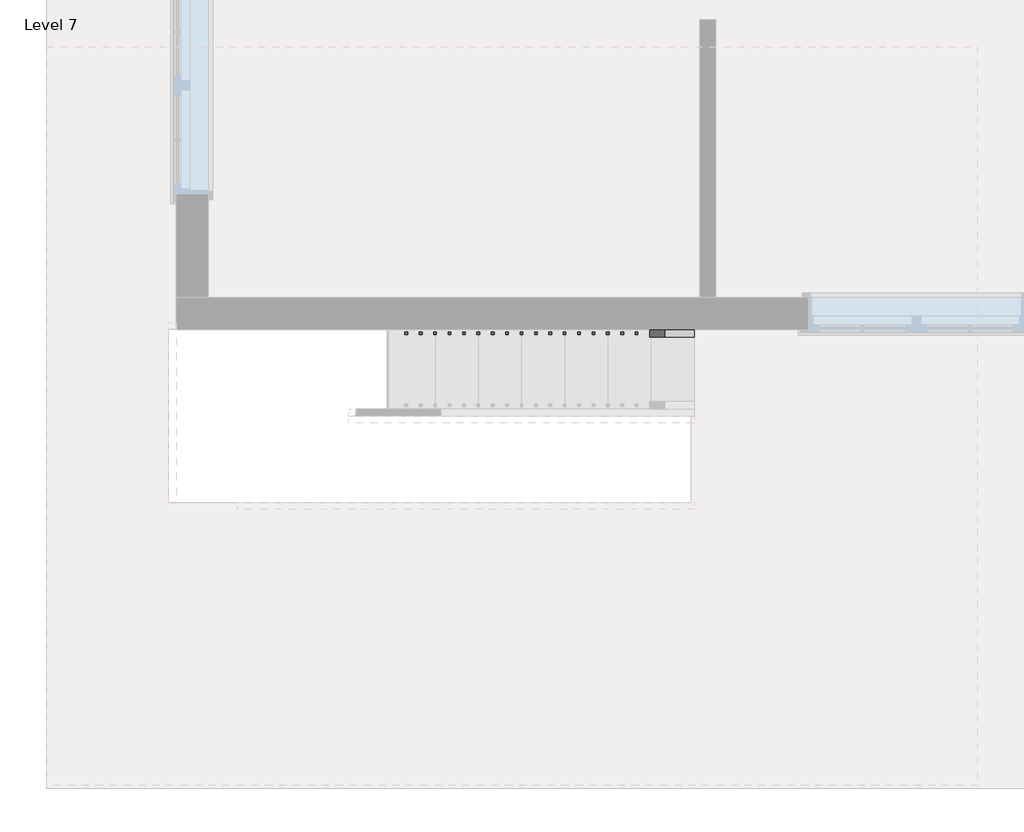
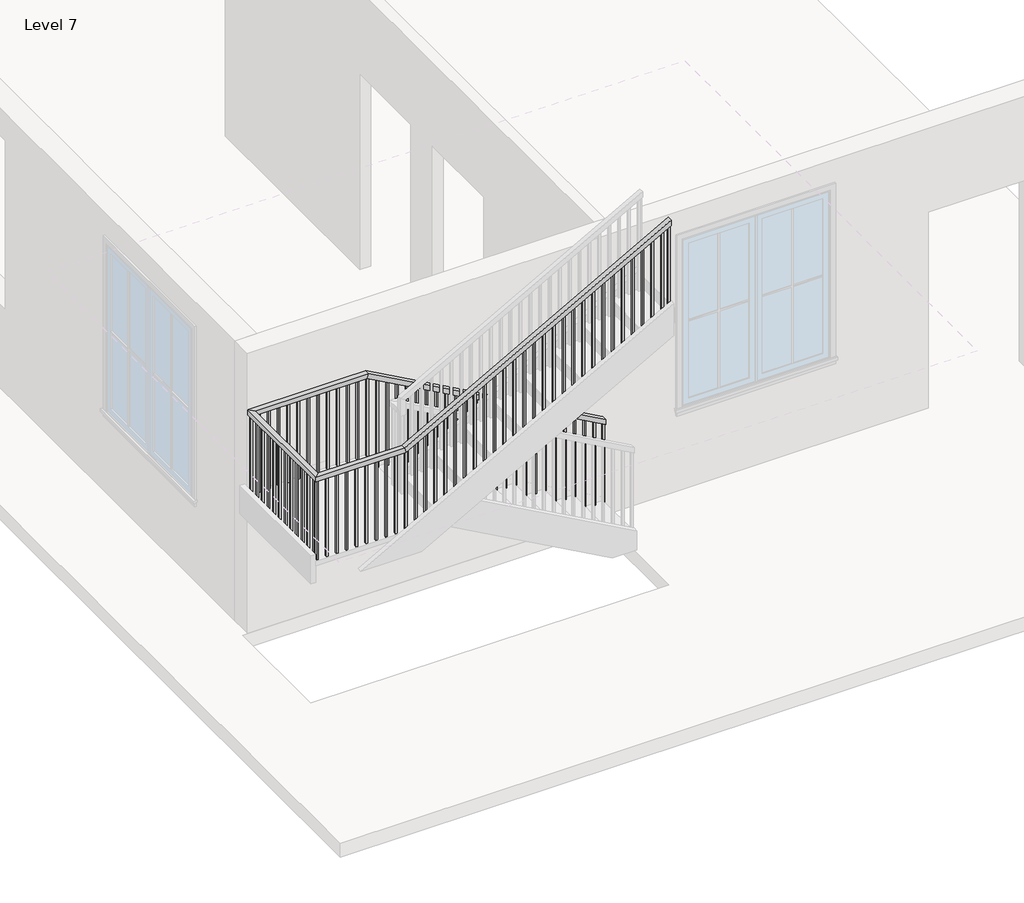
# One storey, part 2 of 3: 1 railing.
"""IFC4 building model written with IfcOpenShell, lengths in millimetres."""

from ifc_helpers import new_model, si_unit, frame, origin, place, context, project, spatial, polyline, outline, extrude, faceted_brep, element, save

model = new_model("IFC4")

# Units and contexts
model_context = context("Model", 3, world=origin())
ifc_project = project(units=[si_unit("LENGTHUNIT", "METRE", prefix="MILLI")], contexts=[model_context])

# Site, building, storey
site = spatial("IfcSite", under=ifc_project)
building = spatial("IfcBuilding", under=site)
storey = spatial("IfcBuildingStorey", under=building, Name="Level 7", Elevation=16002.0)

# Railing
placement = place(None, origin())
element("IfcRailing", 1, ObjectType="Handrail - Rectangular", at=placement, inside=storey, context=model_context, shape_type="SolidModel", body=[
    faceted_brep([(-1805.9198569, -5357.1933037, 17085.7333333), (-1805.9198569, -5357.1933037, 17027.620221), (-1805.9198569, -5306.3933037, 17027.620221), (-1805.9198569, -5306.3933037, 17085.7333333), (-4244.3198569, -5357.1933037, 18440.4), (-4257.4834592, -5357.1933037, 18389.6), (-4257.4834592, -5306.3933037, 18389.6), (-4244.3198569, -5306.3933037, 18440.4), (-5412.7198569, -5357.1933037, 18440.4), (-5412.7198569, -5357.1933037, 18389.6), (-5463.5198569, -5306.3933037, 18389.6), (-5463.5198569, -5306.3933037, 18440.4), (-5412.7198569, -6474.7933037, 18440.4), (-5412.7198569, -6474.7933037, 18389.6), (-5463.5198569, -6525.5933037, 18389.6), (-5463.5198569, -6525.5933037, 18440.4), (-4549.1198569, -6474.7933037, 18440.4), (-4535.9562547, -6474.7933037, 18389.6), (-4535.9562547, -6525.5933037, 18389.6), (-4549.1198569, -6525.5933037, 18440.4), (-1805.9198569, -6474.7933037, 19964.4), (-1805.9198569, -6525.5933037, 19964.4), (-1805.9198569, -6525.5933037, 19906.2868876), (-1805.9198569, -6474.7933037, 19906.2868876)], [[[0, 1, 2, 3]], [[1, 0, 4, 5]], [[2, 1, 5, 6]], [[3, 2, 6, 7]], [[0, 3, 7, 4]], [[5, 4, 8, 9]], [[6, 5, 9, 10]], [[7, 6, 10, 11]], [[4, 7, 11, 8]], [[9, 8, 12, 13]], [[10, 9, 13, 14]], [[11, 10, 14, 15]], [[8, 11, 15, 12]], [[13, 12, 16, 17]], [[14, 13, 17, 18]], [[15, 14, 18, 19]], [[12, 15, 19, 16]], [[20, 21, 22, 23]], [[17, 16, 20, 23]], [[18, 17, 23, 22]], [[19, 18, 22, 21]], [[16, 19, 21, 20]]]),
    extrude(outline(polyline([(19869.245221, -1872.5948569), (19858.6618876, -1891.6448569), (18880.6666667, -1891.6448569), (18880.6666667, -1872.5948569), (19869.245221, -1872.5948569)])), frame((0.0, -6509.7183037, 0.0), z_axis=(0.0, 1.0, 0.0), x_axis=(0.0, 0.0, 1.0)), (0.0, 0.0, 1.0), 19.05),
    extrude(outline(polyline([(19812.8007765, -1974.1948569), (19802.2174432, -1993.2448569), (18880.6666667, -1993.2448569), (18880.6666667, -1974.1948569), (19812.8007765, -1974.1948569)])), frame((0.0, -6509.7183037, 0.0), z_axis=(0.0, 1.0, 0.0), x_axis=(0.0, 0.0, 1.0)), (0.0, 0.0, 1.0), 19.05),
    extrude(outline(polyline([(19756.3563321, -2075.7948569), (19745.7729988, -2094.8448569), (18880.6666667, -2094.8448569), (18880.6666667, -2075.7948569), (19756.3563321, -2075.7948569)])), frame((0.0, -6509.7183037, 0.0), z_axis=(0.0, 1.0, 0.0), x_axis=(0.0, 0.0, 1.0)), (0.0, 0.0, 1.0), 19.05),
    extrude(outline(polyline([(19699.9118876, -2177.3948569), (19689.3285543, -2196.4448569), (18711.3333333, -2196.4448569), (18711.3333333, -2177.3948569), (19699.9118876, -2177.3948569)])), frame((0.0, -6509.7183037, 0.0), z_axis=(0.0, 1.0, 0.0), x_axis=(0.0, 0.0, 1.0)), (0.0, 0.0, 1.0), 19.05),
    extrude(outline(polyline([(19643.4674432, -2278.9948569), (19632.8841099, -2298.0448569), (18711.3333333, -2298.0448569), (18711.3333333, -2278.9948569), (19643.4674432, -2278.9948569)])), frame((0.0, -6509.7183037, 0.0), z_axis=(0.0, 1.0, 0.0), x_axis=(0.0, 0.0, 1.0)), (0.0, 0.0, 1.0), 19.05),
    extrude(outline(polyline([(19587.0229988, -2380.5948569), (19576.4396654, -2399.6448569), (18711.3333333, -2399.6448569), (18711.3333333, -2380.5948569), (19587.0229988, -2380.5948569)])), frame((0.0, -6509.7183037, 0.0), z_axis=(0.0, 1.0, 0.0), x_axis=(0.0, 0.0, 1.0)), (0.0, 0.0, 1.0), 19.05),
    extrude(outline(polyline([(19530.5785543, -2482.1948569), (19519.995221, -2501.2448569), (18542.0, -2501.2448569), (18542.0, -2482.1948569), (19530.5785543, -2482.1948569)])), frame((0.0, -6509.7183037, 0.0), z_axis=(0.0, 1.0, 0.0), x_axis=(0.0, 0.0, 1.0)), (0.0, 0.0, 1.0), 19.05),
    extrude(outline(polyline([(19474.1341099, -2583.7948569), (19463.5507765, -2602.8448569), (18542.0, -2602.8448569), (18542.0, -2583.7948569), (19474.1341099, -2583.7948569)])), frame((0.0, -6509.7183037, 0.0), z_axis=(0.0, 1.0, 0.0), x_axis=(0.0, 0.0, 1.0)), (0.0, 0.0, 1.0), 19.05),
    extrude(outline(polyline([(19417.6896654, -2685.3948569), (19407.1063321, -2704.4448569), (18542.0, -2704.4448569), (18542.0, -2685.3948569), (19417.6896654, -2685.3948569)])), frame((0.0, -6509.7183037, 0.0), z_axis=(0.0, 1.0, 0.0), x_axis=(0.0, 0.0, 1.0)), (0.0, 0.0, 1.0), 19.05),
    extrude(outline(polyline([(19361.245221, -2786.9948569), (19350.6618876, -2806.0448569), (18372.6666667, -2806.0448569), (18372.6666667, -2786.9948569), (19361.245221, -2786.9948569)])), frame((0.0, -6509.7183037, 0.0), z_axis=(0.0, 1.0, 0.0), x_axis=(0.0, 0.0, 1.0)), (0.0, 0.0, 1.0), 19.05),
    extrude(outline(polyline([(19304.8007765, -2888.5948569), (19294.2174432, -2907.6448569), (18372.6666667, -2907.6448569), (18372.6666667, -2888.5948569), (19304.8007765, -2888.5948569)])), frame((0.0, -6509.7183037, 0.0), z_axis=(0.0, 1.0, 0.0), x_axis=(0.0, 0.0, 1.0)), (0.0, 0.0, 1.0), 19.05),
    extrude(outline(polyline([(19248.3563321, -2990.1948569), (19237.7729988, -3009.2448569), (18372.6666667, -3009.2448569), (18372.6666667, -2990.1948569), (19248.3563321, -2990.1948569)])), frame((0.0, -6509.7183037, 0.0), z_axis=(0.0, 1.0, 0.0), x_axis=(0.0, 0.0, 1.0)), (0.0, 0.0, 1.0), 19.05),
    extrude(outline(polyline([(19191.9118876, -3091.7948569), (19181.3285543, -3110.8448569), (18203.3333333, -3110.8448569), (18203.3333333, -3091.7948569), (19191.9118876, -3091.7948569)])), frame((0.0, -6509.7183037, 0.0), z_axis=(0.0, 1.0, 0.0), x_axis=(0.0, 0.0, 1.0)), (0.0, 0.0, 1.0), 19.05),
    extrude(outline(polyline([(19135.4674432, -3193.3948569), (19124.8841099, -3212.4448569), (18203.3333333, -3212.4448569), (18203.3333333, -3193.3948569), (19135.4674432, -3193.3948569)])), frame((0.0, -6509.7183037, 0.0), z_axis=(0.0, 1.0, 0.0), x_axis=(0.0, 0.0, 1.0)), (0.0, 0.0, 1.0), 19.05),
    extrude(outline(polyline([(19079.0229988, -3294.9948569), (19068.4396654, -3314.0448569), (18203.3333333, -3314.0448569), (18203.3333333, -3294.9948569), (19079.0229988, -3294.9948569)])), frame((0.0, -6509.7183037, 0.0), z_axis=(0.0, 1.0, 0.0), x_axis=(0.0, 0.0, 1.0)), (0.0, 0.0, 1.0), 19.05),
    extrude(outline(polyline([(19022.5785543, -3396.5948569), (19011.995221, -3415.6448569), (18034.0, -3415.6448569), (18034.0, -3396.5948569), (19022.5785543, -3396.5948569)])), frame((0.0, -6509.7183037, 0.0), z_axis=(0.0, 1.0, 0.0), x_axis=(0.0, 0.0, 1.0)), (0.0, 0.0, 1.0), 19.05),
    extrude(outline(polyline([(18966.1341099, -3498.1948569), (18955.5507765, -3517.2448569), (18034.0, -3517.2448569), (18034.0, -3498.1948569), (18966.1341099, -3498.1948569)])), frame((0.0, -6509.7183037, 0.0), z_axis=(0.0, 1.0, 0.0), x_axis=(0.0, 0.0, 1.0)), (0.0, 0.0, 1.0), 19.05),
    extrude(outline(polyline([(18909.6896654, -3599.7948569), (18899.1063321, -3618.8448569), (18034.0, -3618.8448569), (18034.0, -3599.7948569), (18909.6896654, -3599.7948569)])), frame((0.0, -6509.7183037, 0.0), z_axis=(0.0, 1.0, 0.0), x_axis=(0.0, 0.0, 1.0)), (0.0, 0.0, 1.0), 19.05),
    extrude(outline(polyline([(18853.245221, -3701.3948569), (18842.6618876, -3720.4448569), (17864.6666667, -3720.4448569), (17864.6666667, -3701.3948569), (18853.245221, -3701.3948569)])), frame((0.0, -6509.7183037, 0.0), z_axis=(0.0, 1.0, 0.0), x_axis=(0.0, 0.0, 1.0)), (0.0, 0.0, 1.0), 19.05),
    extrude(outline(polyline([(18796.8007765, -3802.9948569), (18786.2174432, -3822.0448569), (17864.6666667, -3822.0448569), (17864.6666667, -3802.9948569), (18796.8007765, -3802.9948569)])), frame((0.0, -6509.7183037, 0.0), z_axis=(0.0, 1.0, 0.0), x_axis=(0.0, 0.0, 1.0)), (0.0, 0.0, 1.0), 19.05),
    extrude(outline(polyline([(18740.3563321, -3904.5948569), (18729.7729988, -3923.6448569), (17864.6666667, -3923.6448569), (17864.6666667, -3904.5948569), (18740.3563321, -3904.5948569)])), frame((0.0, -6509.7183037, 0.0), z_axis=(0.0, 1.0, 0.0), x_axis=(0.0, 0.0, 1.0)), (0.0, 0.0, 1.0), 19.05),
    extrude(outline(polyline([(18683.9118876, -4006.1948569), (18673.3285543, -4025.2448569), (17695.3333333, -4025.2448569), (17695.3333333, -4006.1948569), (18683.9118876, -4006.1948569)])), frame((0.0, -6509.7183037, 0.0), z_axis=(0.0, 1.0, 0.0), x_axis=(0.0, 0.0, 1.0)), (0.0, 0.0, 1.0), 19.05),
    extrude(outline(polyline([(18627.4674432, -4107.7948569), (18616.8841099, -4126.8448569), (17695.3333333, -4126.8448569), (17695.3333333, -4107.7948569), (18627.4674432, -4107.7948569)])), frame((0.0, -6509.7183037, 0.0), z_axis=(0.0, 1.0, 0.0), x_axis=(0.0, 0.0, 1.0)), (0.0, 0.0, 1.0), 19.05),
    extrude(outline(polyline([(18571.0229988, -4209.3948569), (18560.4396654, -4228.4448569), (17695.3333333, -4228.4448569), (17695.3333333, -4209.3948569), (18571.0229988, -4209.3948569)])), frame((0.0, -6509.7183037, 0.0), z_axis=(0.0, 1.0, 0.0), x_axis=(0.0, 0.0, 1.0)), (0.0, 0.0, 1.0), 19.05),
    extrude(outline(polyline([(18514.5785543, -4310.9948569), (18503.995221, -4330.0448569), (17526.0, -4330.0448569), (17526.0, -4310.9948569), (18514.5785543, -4310.9948569)])), frame((0.0, -6509.7183037, 0.0), z_axis=(0.0, 1.0, 0.0), x_axis=(0.0, 0.0, 1.0)), (0.0, 0.0, 1.0), 19.05),
    extrude(outline(polyline([(18458.1341099, -4412.5948569), (18447.5507765, -4431.6448569), (17526.0, -4431.6448569), (17526.0, -4412.5948569), (18458.1341099, -4412.5948569)])), frame((0.0, -6509.7183037, 0.0), z_axis=(0.0, 1.0, 0.0), x_axis=(0.0, 0.0, 1.0)), (0.0, 0.0, 1.0), 19.05),
    extrude(outline(polyline([(18401.6896654, -4514.1948569), (18391.1063321, -4533.2448569), (17526.0, -4533.2448569), (17526.0, -4514.1948569), (18401.6896654, -4514.1948569)])), frame((0.0, -6509.7183037, 0.0), z_axis=(0.0, 1.0, 0.0), x_axis=(0.0, 0.0, 1.0)), (0.0, 0.0, 1.0), 19.05),
    extrude(outline(polyline([(-4634.8448569, -6509.7183037), (-4634.8448569, -6490.6683037), (-4615.7948569, -6490.6683037), (-4615.7948569, -6509.7183037), (-4634.8448569, -6509.7183037)])), frame((0.0, 0.0, 17526.0), z_axis=(0.0, 0.0, 1.0), x_axis=(1.0, 0.0, 0.0)), (0.0, 0.0, 1.0), 863.6),
    extrude(outline(polyline([(-4736.4448569, -6509.7183037), (-4736.4448569, -6490.6683037), (-4717.3948569, -6490.6683037), (-4717.3948569, -6509.7183037), (-4736.4448569, -6509.7183037)])), frame((0.0, 0.0, 17526.0), z_axis=(0.0, 0.0, 1.0), x_axis=(1.0, 0.0, 0.0)), (0.0, 0.0, 1.0), 863.6),
    extrude(outline(polyline([(-4838.0448569, -6509.7183037), (-4838.0448569, -6490.6683037), (-4818.9948569, -6490.6683037), (-4818.9948569, -6509.7183037), (-4838.0448569, -6509.7183037)])), frame((0.0, 0.0, 17526.0), z_axis=(0.0, 0.0, 1.0), x_axis=(1.0, 0.0, 0.0)), (0.0, 0.0, 1.0), 863.6),
    extrude(outline(polyline([(-4939.6448569, -6509.7183037), (-4939.6448569, -6490.6683037), (-4920.5948569, -6490.6683037), (-4920.5948569, -6509.7183037), (-4939.6448569, -6509.7183037)])), frame((0.0, 0.0, 17526.0), z_axis=(0.0, 0.0, 1.0), x_axis=(1.0, 0.0, 0.0)), (0.0, 0.0, 1.0), 863.6),
    extrude(outline(polyline([(-5041.2448569, -6509.7183037), (-5041.2448569, -6490.6683037), (-5022.1948569, -6490.6683037), (-5022.1948569, -6509.7183037), (-5041.2448569, -6509.7183037)])), frame((0.0, 0.0, 17526.0), z_axis=(0.0, 0.0, 1.0), x_axis=(1.0, 0.0, 0.0)), (0.0, 0.0, 1.0), 863.6),
    extrude(outline(polyline([(-5142.8448569, -6509.7183037), (-5142.8448569, -6490.6683037), (-5123.7948569, -6490.6683037), (-5123.7948569, -6509.7183037), (-5142.8448569, -6509.7183037)])), frame((0.0, 0.0, 17526.0), z_axis=(0.0, 0.0, 1.0), x_axis=(1.0, 0.0, 0.0)), (0.0, 0.0, 1.0), 863.6),
    extrude(outline(polyline([(-5244.4448569, -6509.7183037), (-5244.4448569, -6490.6683037), (-5225.3948569, -6490.6683037), (-5225.3948569, -6509.7183037), (-5244.4448569, -6509.7183037)])), frame((0.0, 0.0, 17526.0), z_axis=(0.0, 0.0, 1.0), x_axis=(1.0, 0.0, 0.0)), (0.0, 0.0, 1.0), 863.6),
    extrude(outline(polyline([(-5346.0448569, -6509.7183037), (-5346.0448569, -6490.6683037), (-5326.9948569, -6490.6683037), (-5326.9948569, -6509.7183037), (-5346.0448569, -6509.7183037)])), frame((0.0, 0.0, 17526.0), z_axis=(0.0, 0.0, 1.0), x_axis=(1.0, 0.0, 0.0)), (0.0, 0.0, 1.0), 863.6),
    extrude(outline(polyline([(-5447.6448569, -6439.8683037), (-5428.5948569, -6439.8683037), (-5428.5948569, -6458.9183037), (-5447.6448569, -6458.9183037), (-5447.6448569, -6439.8683037)])), frame((0.0, 0.0, 17526.0), z_axis=(0.0, 0.0, 1.0), x_axis=(1.0, 0.0, 0.0)), (0.0, 0.0, 1.0), 863.6),
    extrude(outline(polyline([(-5447.6448569, -6338.2683037), (-5428.5948569, -6338.2683037), (-5428.5948569, -6357.3183037), (-5447.6448569, -6357.3183037), (-5447.6448569, -6338.2683037)])), frame((0.0, 0.0, 17526.0), z_axis=(0.0, 0.0, 1.0), x_axis=(1.0, 0.0, 0.0)), (0.0, 0.0, 1.0), 863.6),
    extrude(outline(polyline([(-5447.6448569, -6236.6683037), (-5428.5948569, -6236.6683037), (-5428.5948569, -6255.7183037), (-5447.6448569, -6255.7183037), (-5447.6448569, -6236.6683037)])), frame((0.0, 0.0, 17526.0), z_axis=(0.0, 0.0, 1.0), x_axis=(1.0, 0.0, 0.0)), (0.0, 0.0, 1.0), 863.6),
    extrude(outline(polyline([(-5447.6448569, -6135.0683037), (-5428.5948569, -6135.0683037), (-5428.5948569, -6154.1183037), (-5447.6448569, -6154.1183037), (-5447.6448569, -6135.0683037)])), frame((0.0, 0.0, 17526.0), z_axis=(0.0, 0.0, 1.0), x_axis=(1.0, 0.0, 0.0)), (0.0, 0.0, 1.0), 863.6),
    extrude(outline(polyline([(-5447.6448569, -6033.4683037), (-5428.5948569, -6033.4683037), (-5428.5948569, -6052.5183037), (-5447.6448569, -6052.5183037), (-5447.6448569, -6033.4683037)])), frame((0.0, 0.0, 17526.0), z_axis=(0.0, 0.0, 1.0), x_axis=(1.0, 0.0, 0.0)), (0.0, 0.0, 1.0), 863.6),
    extrude(outline(polyline([(-5447.6448569, -5931.8683037), (-5428.5948569, -5931.8683037), (-5428.5948569, -5950.9183037), (-5447.6448569, -5950.9183037), (-5447.6448569, -5931.8683037)])), frame((0.0, 0.0, 17526.0), z_axis=(0.0, 0.0, 1.0), x_axis=(1.0, 0.0, 0.0)), (0.0, 0.0, 1.0), 863.6),
    extrude(outline(polyline([(-5447.6448569, -5830.2683037), (-5428.5948569, -5830.2683037), (-5428.5948569, -5849.3183037), (-5447.6448569, -5849.3183037), (-5447.6448569, -5830.2683037)])), frame((0.0, 0.0, 17526.0), z_axis=(0.0, 0.0, 1.0), x_axis=(1.0, 0.0, 0.0)), (0.0, 0.0, 1.0), 863.6),
    extrude(outline(polyline([(-5447.6448569, -5728.6683037), (-5428.5948569, -5728.6683037), (-5428.5948569, -5747.7183037), (-5447.6448569, -5747.7183037), (-5447.6448569, -5728.6683037)])), frame((0.0, 0.0, 17526.0), z_axis=(0.0, 0.0, 1.0), x_axis=(1.0, 0.0, 0.0)), (0.0, 0.0, 1.0), 863.6),
    extrude(outline(polyline([(-5447.6448569, -5627.0683037), (-5428.5948569, -5627.0683037), (-5428.5948569, -5646.1183037), (-5447.6448569, -5646.1183037), (-5447.6448569, -5627.0683037)])), frame((0.0, 0.0, 17526.0), z_axis=(0.0, 0.0, 1.0), x_axis=(1.0, 0.0, 0.0)), (0.0, 0.0, 1.0), 863.6),
    extrude(outline(polyline([(-5447.6448569, -5525.4683037), (-5428.5948569, -5525.4683037), (-5428.5948569, -5544.5183037), (-5447.6448569, -5544.5183037), (-5447.6448569, -5525.4683037)])), frame((0.0, 0.0, 17526.0), z_axis=(0.0, 0.0, 1.0), x_axis=(1.0, 0.0, 0.0)), (0.0, 0.0, 1.0), 863.6),
    extrude(outline(polyline([(-5447.6448569, -5423.8683037), (-5428.5948569, -5423.8683037), (-5428.5948569, -5442.9183037), (-5447.6448569, -5442.9183037), (-5447.6448569, -5423.8683037)])), frame((0.0, 0.0, 17526.0), z_axis=(0.0, 0.0, 1.0), x_axis=(1.0, 0.0, 0.0)), (0.0, 0.0, 1.0), 863.6),
    extrude(outline(polyline([(-5352.3948569, -5322.2683037), (-5352.3948569, -5341.3183037), (-5371.4448569, -5341.3183037), (-5371.4448569, -5322.2683037), (-5352.3948569, -5322.2683037)])), frame((0.0, 0.0, 17526.0), z_axis=(0.0, 0.0, 1.0), x_axis=(1.0, 0.0, 0.0)), (0.0, 0.0, 1.0), 863.6),
    extrude(outline(polyline([(-5250.7948569, -5322.2683037), (-5250.7948569, -5341.3183037), (-5269.8448569, -5341.3183037), (-5269.8448569, -5322.2683037), (-5250.7948569, -5322.2683037)])), frame((0.0, 0.0, 17526.0), z_axis=(0.0, 0.0, 1.0), x_axis=(1.0, 0.0, 0.0)), (0.0, 0.0, 1.0), 863.6),
    extrude(outline(polyline([(-5149.1948569, -5322.2683037), (-5149.1948569, -5341.3183037), (-5168.2448569, -5341.3183037), (-5168.2448569, -5322.2683037), (-5149.1948569, -5322.2683037)])), frame((0.0, 0.0, 17526.0), z_axis=(0.0, 0.0, 1.0), x_axis=(1.0, 0.0, 0.0)), (0.0, 0.0, 1.0), 863.6),
    extrude(outline(polyline([(-5047.5948569, -5322.2683037), (-5047.5948569, -5341.3183037), (-5066.6448569, -5341.3183037), (-5066.6448569, -5322.2683037), (-5047.5948569, -5322.2683037)])), frame((0.0, 0.0, 17526.0), z_axis=(0.0, 0.0, 1.0), x_axis=(1.0, 0.0, 0.0)), (0.0, 0.0, 1.0), 863.6),
    extrude(outline(polyline([(-4945.9948569, -5322.2683037), (-4945.9948569, -5341.3183037), (-4965.0448569, -5341.3183037), (-4965.0448569, -5322.2683037), (-4945.9948569, -5322.2683037)])), frame((0.0, 0.0, 17526.0), z_axis=(0.0, 0.0, 1.0), x_axis=(1.0, 0.0, 0.0)), (0.0, 0.0, 1.0), 863.6),
    extrude(outline(polyline([(-4844.3948569, -5322.2683037), (-4844.3948569, -5341.3183037), (-4863.4448569, -5341.3183037), (-4863.4448569, -5322.2683037), (-4844.3948569, -5322.2683037)])), frame((0.0, 0.0, 17526.0), z_axis=(0.0, 0.0, 1.0), x_axis=(1.0, 0.0, 0.0)), (0.0, 0.0, 1.0), 863.6),
    extrude(outline(polyline([(-4742.7948569, -5322.2683037), (-4742.7948569, -5341.3183037), (-4761.8448569, -5341.3183037), (-4761.8448569, -5322.2683037), (-4742.7948569, -5322.2683037)])), frame((0.0, 0.0, 17526.0), z_axis=(0.0, 0.0, 1.0), x_axis=(1.0, 0.0, 0.0)), (0.0, 0.0, 1.0), 863.6),
    extrude(outline(polyline([(-4641.1948569, -5322.2683037), (-4641.1948569, -5341.3183037), (-4660.2448569, -5341.3183037), (-4660.2448569, -5322.2683037), (-4641.1948569, -5322.2683037)])), frame((0.0, 0.0, 17526.0), z_axis=(0.0, 0.0, 1.0), x_axis=(1.0, 0.0, 0.0)), (0.0, 0.0, 1.0), 863.6),
    extrude(outline(polyline([(-4539.5948569, -5322.2683037), (-4539.5948569, -5341.3183037), (-4558.6448569, -5341.3183037), (-4558.6448569, -5322.2683037), (-4539.5948569, -5322.2683037)])), frame((0.0, 0.0, 17526.0), z_axis=(0.0, 0.0, 1.0), x_axis=(1.0, 0.0, 0.0)), (0.0, 0.0, 1.0), 863.6),
    extrude(outline(polyline([(-4437.9948569, -5322.2683037), (-4437.9948569, -5341.3183037), (-4457.0448569, -5341.3183037), (-4457.0448569, -5322.2683037), (-4437.9948569, -5322.2683037)])), frame((0.0, 0.0, 17526.0), z_axis=(0.0, 0.0, 1.0), x_axis=(1.0, 0.0, 0.0)), (0.0, 0.0, 1.0), 863.6),
    extrude(outline(polyline([(-4336.3948569, -5322.2683037), (-4336.3948569, -5341.3183037), (-4355.4448569, -5341.3183037), (-4355.4448569, -5322.2683037), (-4336.3948569, -5322.2683037)])), frame((0.0, 0.0, 17526.0), z_axis=(0.0, 0.0, 1.0), x_axis=(1.0, 0.0, 0.0)), (0.0, 0.0, 1.0), 863.6),
    extrude(outline(polyline([(18376.995221, -4234.7948569), (18387.5785543, -4253.8448569), (17526.0, -4253.8448569), (17526.0, -4234.7948569), (18376.995221, -4234.7948569)])), frame((0.0, -5341.3183037, 0.0), z_axis=(0.0, 1.0, 0.0), x_axis=(0.0, 0.0, 1.0)), (0.0, 0.0, 1.0), 19.05),
    extrude(outline(polyline([(18320.5507765, -4133.1948569), (18331.1341099, -4152.2448569), (17356.6666667, -4152.2448569), (17356.6666667, -4133.1948569), (18320.5507765, -4133.1948569)])), frame((0.0, -5341.3183037, 0.0), z_axis=(0.0, 1.0, 0.0), x_axis=(0.0, 0.0, 1.0)), (0.0, 0.0, 1.0), 19.05),
    extrude(outline(polyline([(18264.1063321, -4031.5948569), (18274.6896654, -4050.6448569), (17356.6666667, -4050.6448569), (17356.6666667, -4031.5948569), (18264.1063321, -4031.5948569)])), frame((0.0, -5341.3183037, 0.0), z_axis=(0.0, 1.0, 0.0), x_axis=(0.0, 0.0, 1.0)), (0.0, 0.0, 1.0), 19.05),
    extrude(outline(polyline([(18207.6618876, -3929.9948569), (18218.245221, -3949.0448569), (17356.6666667, -3949.0448569), (17356.6666667, -3929.9948569), (18207.6618876, -3929.9948569)])), frame((0.0, -5341.3183037, 0.0), z_axis=(0.0, 1.0, 0.0), x_axis=(0.0, 0.0, 1.0)), (0.0, 0.0, 1.0), 19.05),
    extrude(outline(polyline([(18151.2174432, -3828.3948569), (18161.8007765, -3847.4448569), (17187.3333333, -3847.4448569), (17187.3333333, -3828.3948569), (18151.2174432, -3828.3948569)])), frame((0.0, -5341.3183037, 0.0), z_axis=(0.0, 1.0, 0.0), x_axis=(0.0, 0.0, 1.0)), (0.0, 0.0, 1.0), 19.05),
    extrude(outline(polyline([(18094.7729988, -3726.7948569), (18105.3563321, -3745.8448569), (17187.3333333, -3745.8448569), (17187.3333333, -3726.7948569), (18094.7729988, -3726.7948569)])), frame((0.0, -5341.3183037, 0.0), z_axis=(0.0, 1.0, 0.0), x_axis=(0.0, 0.0, 1.0)), (0.0, 0.0, 1.0), 19.05),
    extrude(outline(polyline([(18038.3285543, -3625.1948569), (18048.9118876, -3644.2448569), (17187.3333333, -3644.2448569), (17187.3333333, -3625.1948569), (18038.3285543, -3625.1948569)])), frame((0.0, -5341.3183037, 0.0), z_axis=(0.0, 1.0, 0.0), x_axis=(0.0, 0.0, 1.0)), (0.0, 0.0, 1.0), 19.05),
    extrude(outline(polyline([(17981.8841099, -3523.5948569), (17992.4674432, -3542.6448569), (17018.0, -3542.6448569), (17018.0, -3523.5948569), (17981.8841099, -3523.5948569)])), frame((0.0, -5341.3183037, 0.0), z_axis=(0.0, 1.0, 0.0), x_axis=(0.0, 0.0, 1.0)), (0.0, 0.0, 1.0), 19.05),
    extrude(outline(polyline([(17925.4396654, -3421.9948569), (17936.0229988, -3441.0448569), (17018.0, -3441.0448569), (17018.0, -3421.9948569), (17925.4396654, -3421.9948569)])), frame((0.0, -5341.3183037, 0.0), z_axis=(0.0, 1.0, 0.0), x_axis=(0.0, 0.0, 1.0)), (0.0, 0.0, 1.0), 19.05),
    extrude(outline(polyline([(17868.995221, -3320.3948569), (17879.5785543, -3339.4448569), (17018.0, -3339.4448569), (17018.0, -3320.3948569), (17868.995221, -3320.3948569)])), frame((0.0, -5341.3183037, 0.0), z_axis=(0.0, 1.0, 0.0), x_axis=(0.0, 0.0, 1.0)), (0.0, 0.0, 1.0), 19.05),
    extrude(outline(polyline([(17812.5507765, -3218.7948569), (17823.1341099, -3237.8448569), (16848.6666667, -3237.8448569), (16848.6666667, -3218.7948569), (17812.5507765, -3218.7948569)])), frame((0.0, -5341.3183037, 0.0), z_axis=(0.0, 1.0, 0.0), x_axis=(0.0, 0.0, 1.0)), (0.0, 0.0, 1.0), 19.05),
    extrude(outline(polyline([(17756.1063321, -3117.1948569), (17766.6896654, -3136.2448569), (16848.6666667, -3136.2448569), (16848.6666667, -3117.1948569), (17756.1063321, -3117.1948569)])), frame((0.0, -5341.3183037, 0.0), z_axis=(0.0, 1.0, 0.0), x_axis=(0.0, 0.0, 1.0)), (0.0, 0.0, 1.0), 19.05),
    extrude(outline(polyline([(17699.6618876, -3015.5948569), (17710.245221, -3034.6448569), (16848.6666667, -3034.6448569), (16848.6666667, -3015.5948569), (17699.6618876, -3015.5948569)])), frame((0.0, -5341.3183037, 0.0), z_axis=(0.0, 1.0, 0.0), x_axis=(0.0, 0.0, 1.0)), (0.0, 0.0, 1.0), 19.05),
    extrude(outline(polyline([(17643.2174432, -2913.9948569), (17653.8007765, -2933.0448569), (16679.3333333, -2933.0448569), (16679.3333333, -2913.9948569), (17643.2174432, -2913.9948569)])), frame((0.0, -5341.3183037, 0.0), z_axis=(0.0, 1.0, 0.0), x_axis=(0.0, 0.0, 1.0)), (0.0, 0.0, 1.0), 19.05),
    extrude(outline(polyline([(17586.7729988, -2812.3948569), (17597.3563321, -2831.4448569), (16679.3333333, -2831.4448569), (16679.3333333, -2812.3948569), (17586.7729988, -2812.3948569)])), frame((0.0, -5341.3183037, 0.0), z_axis=(0.0, 1.0, 0.0), x_axis=(0.0, 0.0, 1.0)), (0.0, 0.0, 1.0), 19.05),
    extrude(outline(polyline([(17530.3285543, -2710.7948569), (17540.9118876, -2729.8448569), (16679.3333333, -2729.8448569), (16679.3333333, -2710.7948569), (17530.3285543, -2710.7948569)])), frame((0.0, -5341.3183037, 0.0), z_axis=(0.0, 1.0, 0.0), x_axis=(0.0, 0.0, 1.0)), (0.0, 0.0, 1.0), 19.05),
    extrude(outline(polyline([(17473.8841099, -2609.1948569), (17484.4674432, -2628.2448569), (16510.0, -2628.2448569), (16510.0, -2609.1948569), (17473.8841099, -2609.1948569)])), frame((0.0, -5341.3183037, 0.0), z_axis=(0.0, 1.0, 0.0), x_axis=(0.0, 0.0, 1.0)), (0.0, 0.0, 1.0), 19.05),
    extrude(outline(polyline([(17417.4396654, -2507.5948569), (17428.0229988, -2526.6448569), (16510.0, -2526.6448569), (16510.0, -2507.5948569), (17417.4396654, -2507.5948569)])), frame((0.0, -5341.3183037, 0.0), z_axis=(0.0, 1.0, 0.0), x_axis=(0.0, 0.0, 1.0)), (0.0, 0.0, 1.0), 19.05),
    extrude(outline(polyline([(17360.995221, -2405.9948569), (17371.5785543, -2425.0448569), (16510.0, -2425.0448569), (16510.0, -2405.9948569), (17360.995221, -2405.9948569)])), frame((0.0, -5341.3183037, 0.0), z_axis=(0.0, 1.0, 0.0), x_axis=(0.0, 0.0, 1.0)), (0.0, 0.0, 1.0), 19.05),
    extrude(outline(polyline([(17304.5507765, -2304.3948569), (17315.1341099, -2323.4448569), (16340.6666667, -2323.4448569), (16340.6666667, -2304.3948569), (17304.5507765, -2304.3948569)])), frame((0.0, -5341.3183037, 0.0), z_axis=(0.0, 1.0, 0.0), x_axis=(0.0, 0.0, 1.0)), (0.0, 0.0, 1.0), 19.05),
    extrude(outline(polyline([(17248.1063321, -2202.7948569), (17258.6896654, -2221.8448569), (16340.6666667, -2221.8448569), (16340.6666667, -2202.7948569), (17248.1063321, -2202.7948569)])), frame((0.0, -5341.3183037, 0.0), z_axis=(0.0, 1.0, 0.0), x_axis=(0.0, 0.0, 1.0)), (0.0, 0.0, 1.0), 19.05),
    extrude(outline(polyline([(17191.6618876, -2101.1948569), (17202.245221, -2120.2448569), (16340.6666667, -2120.2448569), (16340.6666667, -2101.1948569), (17191.6618876, -2101.1948569)])), frame((0.0, -5341.3183037, 0.0), z_axis=(0.0, 1.0, 0.0), x_axis=(0.0, 0.0, 1.0)), (0.0, 0.0, 1.0), 19.05),
    extrude(outline(polyline([(17135.2174432, -1999.5948569), (17145.8007765, -2018.6448569), (16171.3333333, -2018.6448569), (16171.3333333, -1999.5948569), (17135.2174432, -1999.5948569)])), frame((0.0, -5341.3183037, 0.0), z_axis=(0.0, 1.0, 0.0), x_axis=(0.0, 0.0, 1.0)), (0.0, 0.0, 1.0), 19.05),
    extrude(outline(polyline([(17078.7729988, -1897.9948569), (17089.3563321, -1917.0448569), (16171.3333333, -1917.0448569), (16171.3333333, -1897.9948569), (17078.7729988, -1897.9948569)])), frame((0.0, -5341.3183037, 0.0), z_axis=(0.0, 1.0, 0.0), x_axis=(0.0, 0.0, 1.0)), (0.0, 0.0, 1.0), 19.05),
    extrude(outline(polyline([(-5447.6448569, -6490.6683037), (-5428.5948569, -6490.6683037), (-5428.5948569, -6509.7183037), (-5447.6448569, -6509.7183037), (-5447.6448569, -6490.6683037)])), frame((0.0, 0.0, 17526.0), z_axis=(0.0, 0.0, 1.0), x_axis=(1.0, 0.0, 0.0)), (0.0, 0.0, 1.0), 863.6),
    extrude(outline(polyline([(-5428.5948569, -5322.2683037), (-5428.5948569, -5341.3183037), (-5447.6448569, -5341.3183037), (-5447.6448569, -5322.2683037), (-5428.5948569, -5322.2683037)])), frame((0.0, 0.0, 17526.0), z_axis=(0.0, 0.0, 1.0), x_axis=(1.0, 0.0, 0.0)), (0.0, 0.0, 1.0), 863.6),
    extrude(outline(polyline([(19906.2868876, -1805.9198569), (19895.7035543, -1824.9698569), (18880.6666667, -1824.9698569), (18880.6666667, -1805.9198569), (19906.2868876, -1805.9198569)])), frame((0.0, -6509.7183037, 0.0), z_axis=(0.0, 1.0, 0.0), x_axis=(0.0, 0.0, 1.0)), (0.0, 0.0, 1.0), 19.05),
    extrude(outline(polyline([(17027.620221, -1805.9198569), (17038.2035543, -1824.9698569), (16171.3333333, -1824.9698569), (16171.3333333, -1805.9198569), (17027.620221, -1805.9198569)])), frame((0.0, -5341.3183037, 0.0), z_axis=(0.0, 1.0, 0.0), x_axis=(0.0, 0.0, 1.0)), (0.0, 0.0, 1.0), 19.05),
])

save(model, "model.ifc")

# Revit data of these elements
# Type "Handrail - Rectangular"
#   Assembly Code = "C2010400"
#   built-in parameter 1008612 = 0.0416667 (stored number, unit not read)
#   built-in parameter 1008611 = 0.0416667 (stored number, unit not read)
#   built-in parameter 1008609 = 0.333333 (stored number, unit not read)
#   built-in parameter 1008604 = 0.166667 (stored number, unit not read)
#   built-in parameter 1008603 = 0.166667 (stored number, unit not read)
#   Railing Height = 3' - 0"
#   built-in parameter 1008630 = 2
#   built-in parameter 1008610 = 2
#   built-in parameter 1008618 = Baluster - Square : 3/4"
# Element 1 (IfcRailing, "Handrail - Rectangular")
#   Phase Created = New Construction
